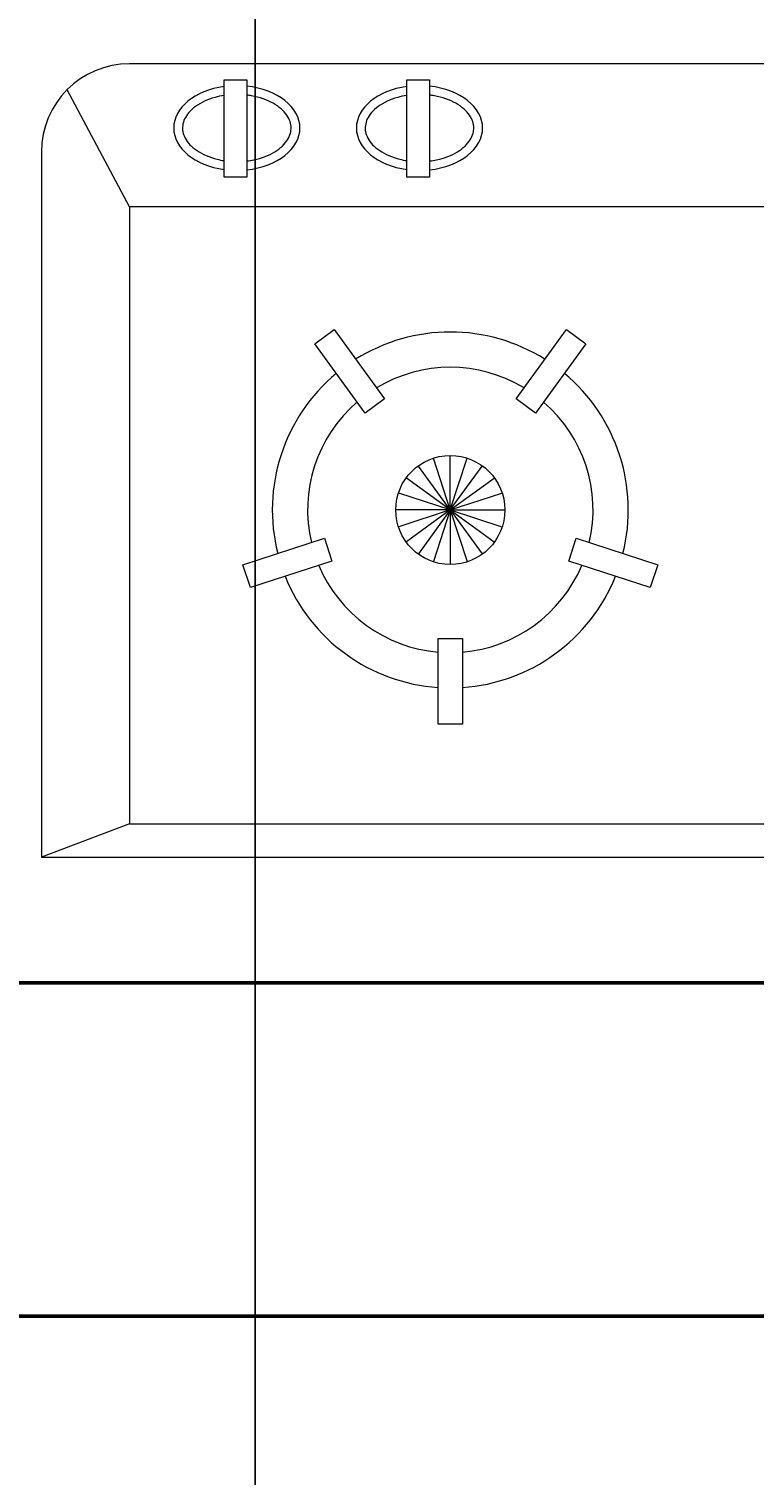
# Model space of a CAD drawing. Units: inches. Extents: x -173 to 545, y -746 to 104.
# Tile 10 of 32: x 300 to 320, y -702 to -663. Entities that reach past the tile are written whole.
import ezdxf

# ---------------------------------------------------------------- set-up
doc = ezdxf.new("R2010")
doc.units = ezdxf.units.IN
doc.header["$MEASUREMENT"] = 0
for name, color, linetype, lineweight in [('A-ANNO-DIMS', 2, 'Continuous', 18), ('A-EQPM', 8, 'Continuous', 18), ('A-WALL', 7, 'Continuous', 50)]:
    doc.layers.add(name, color=color, linetype=linetype, lineweight=lineweight)
doc.styles.get("Standard").update_dxf_attribs({"font": 'arial.ttf'})
doc.dimstyles.get("Standard").update_dxf_attribs({"dimtxt": 0.18, "dimasz": 0.18, "dimexe": 0.18, "dimexo": 0.0625, "dimgap": 0.09, "dimtad": 0, "dimtih": 1, "dimtoh": 1, "dimdec": 0, "dimzin": 0, "dimdsep": 46, "dimlunit": 3, "dimtxsty": 'Standard', "dimcen": 0.09, "dimadec": 0, "dimazin": 0, "dimtfac": 1, "dimtdec": 0, "dimtofl": 0, "dimtmove": 0, "dimatfit": 3, "dimfxl": 1, "dimtolj": 1, "dimtzin": 0, "dimarcsym": 0})

# ---------------------------------------------------------------- blocks, each defined once
blk = doc.blocks.new('HOB-38-BURNER')
for p, q in [((1.939, 10.273), (2.465, 10.656)), ((2.465, 10.656), (3.825, 8.784)), ((7.38, 8.784), (8.739, 10.656)), ((8.739, 10.656), (9.265, 10.273)), ((3.299, 8.402), (1.939, 10.273)), ((9.265, 10.273), (7.906, 8.402)), ((3.825, 8.784), (3.299, 8.402)), ((7.906, 8.402), (7.38, 8.784)), ((5.602, 5.784), (5.149, 7.18)), ((5.602, 5.784), (5.602, 7.251)), ((5.602, 5.784), (6.056, 7.18)), ((5.602, 5.784), (4.415, 6.647)), ((5.602, 5.784), (4.74, 6.971)), ((5.602, 5.784), (6.465, 6.971)), ((5.602, 5.784), (6.789, 6.647)), ((5.602, 5.784), (4.207, 6.238)), ((5.602, 5.784), (6.997, 6.238)), ((5.602, 5.784), (4.135, 5.784)), ((5.602, 5.784), (4.207, 5.331)), ((5.602, 5.784), (4.415, 4.922)), ((5.602, 5.784), (4.74, 4.598)), ((5.602, 5.784), (5.149, 4.389)), ((5.602, 5.784), (7.069, 5.784)), ((5.602, 5.784), (6.997, 5.331)), ((5.602, 5.784), (6.789, 4.922)), ((5.602, 5.784), (6.465, 4.598)), ((5.602, 5.784), (6.056, 4.389)), ((5.602, 5.784), (5.602, 4.317)), ((0, 4.306), (2.2, 5.021)), ((2.2, 5.021), (2.401, 4.402)), ((8.804, 4.402), (9.005, 5.021)), ((9.005, 5.021), (11.204, 4.306)), ((0.201, 3.688), (0, 4.306)), ((2.401, 4.402), (0.201, 3.688)), ((11.003, 3.688), (8.804, 4.402)), ((11.204, 4.306), (11.003, 3.688)), ((5.277, 2.313), (5.927, 2.313)), ((5.277, 0), (5.277, 2.313)), ((5.927, 2.313), (5.927, 0)), ((5.927, 0), (5.277, 0))]:
    blk.add_line(p, q)
blk.add_circle((5.602, 5.784), 1.474)
for radius, start, end in [(4.808, 57.8765, 122.1235), (4.808, 129.8765, 194.1235), (3.855, 58.8365, 121.1635), (4.808, 345.8765, 50.1235), (3.855, 130.8365, 193.1635), (3.855, 346.8365, 49.1635), (4.808, 201.8765, 266.1235), (3.855, 202.8365, 265.1635), (3.855, 274.8365, 337.1635), (4.808, 273.8765, 338.1235)]:
    blk.add_arc((5.602, 5.784), radius, start, end)
blk = doc.blocks.new('*D81')
at = {"layer": 'A-ANNO-DIMS', "color": 0, "lineweight": -2, "transparency": 16777216}
for p, q in [((219.801, -551.924), (219.801, -740.642)), ((306.301, -551.924), (306.301, -740.642)), ((219.981, -740.462), (262.513, -740.462)), ((306.121, -740.462), (263.59, -740.462))]:
    blk.add_line(p, q, dxfattribs=at)
at = {"layer": 'A-ANNO-DIMS', "color": 0, "transparency": 16777216}
for points in [[(219.981, -740.432), (219.981, -740.492), (219.801, -740.462)], [(306.121, -740.432), (306.121, -740.492), (306.301, -740.462)]]:
    blk.add_solid(points, dxfattribs=at)
at = {"layer": 'Defpoints', "color": 0, "transparency": 16777216}
for p in [(219.801, -551.862), (306.301, -551.862), (306.301, -740.462)]:
    blk.add_point(p, dxfattribs=at)
at = {"layer": 'A-ANNO-DIMS', "color": 0, "transparency": 16777216, "insert": (263.051, -740.462), "char_height": 0.18, "attachment_point": 5}
blk.add_mtext('\\A1;7\'-2 1/2"', dxfattribs=at)

msp = doc.modelspace()

# ---------------------------------------------------------------- linework, layer by layer
at = {"layer": 'A-EQPM'}
for p, q in [((336.255, -663.529), (302.912, -663.529)), ((302.912, -667.388), (301.227, -664.227)), ((305.464, -666.593), (305.464, -663.958)), ((305.464, -663.958), (306.08, -663.958)), ((306.08, -663.958), (306.08, -666.593)), ((310.398, -666.593), (310.398, -663.958)), ((310.398, -663.958), (311.015, -663.958)), ((311.015, -663.958), (311.015, -666.593)), ((300.53, -665.911), (300.53, -684.964)), ((306.08, -666.593), (305.464, -666.593)), ((311.015, -666.593), (310.398, -666.593)), ((302.912, -667.388), (302.912, -684.059)), ((336.255, -667.388), (302.912, -667.388)), ((302.912, -684.059), (300.53, -684.964)), ((302.912, -684.059), (336.255, -684.059)), ((300.53, -684.964), (338.637, -684.964))]:
    msp.add_line(p, q, dxfattribs=at)
msp.add_arc((302.912, -665.911), 2.382, 90, 180, dxfattribs=at)
for centre, major_axis, start_param, end_param in [((305.809, -665.263), (1.705, 0), 1.774361, 4.508825), ((305.809, -665.263), (-1.705, 0), 1.73081, 4.552375), ((310.743, -665.263), (1.705, 0), 1.774361, 4.508825), ((310.743, -665.263), (-1.705, 0), 1.73081, 4.552375)]:
    msp.add_ellipse(centre, major_axis=major_axis, ratio=0.671641, start_param=start_param, end_param=end_param, dxfattribs=at)
for points, knots in [([(305.464, -664.383), (305.381, -664.395), (305.3, -664.413), (305.119, -664.463), (305.022, -664.499), (304.845, -664.582), (304.764, -664.629), (304.623, -664.732), (304.563, -664.788), (304.465, -664.902), (304.427, -664.961), (304.371, -665.077), (304.354, -665.135), (304.339, -665.251), (304.341, -665.308), (304.363, -665.423), (304.384, -665.482), (304.447, -665.598), (304.489, -665.657), (304.596, -665.769), (304.66, -665.824), (304.808, -665.924), (304.892, -665.969), (305.075, -666.048), (305.175, -666.081), (305.339, -666.122), (305.401, -666.134), (305.464, -666.144)], [8.079302, 8.079302, 8.079302, 8.079302, 8.245651, 8.245651, 8.463703, 8.463703, 8.681755, 8.681755, 8.899807, 8.899807, 9.117859, 9.117859, 9.33591, 9.33591, 9.553962, 9.553962, 9.772014, 9.772014, 9.990066, 9.990066, 10.208118, 10.208118, 10.426169, 10.426169, 10.644221, 10.644221, 10.770253, 10.770253, 10.770253, 10.770253]), ([(306.08, -666.154), (306.144, -666.146), (306.207, -666.136), (306.375, -666.101), (306.477, -666.071), (306.666, -665.998), (306.754, -665.954), (306.911, -665.859), (306.98, -665.806), (307.096, -665.695), (307.143, -665.637), (307.216, -665.521), (307.241, -665.462), (307.269, -665.357), (307.275, -665.31), (307.275, -665.263), (307.275, -665.206), (307.266, -665.148), (307.228, -665.032), (307.199, -664.973), (307.118, -664.857), (307.067, -664.8), (306.943, -664.691), (306.87, -664.64), (306.706, -664.548), (306.616, -664.507), (306.421, -664.439), (306.317, -664.411), (306.167, -664.384), (306.124, -664.378), (306.08, -664.373)], [4.889299, 4.889299, 4.889299, 4.889299, 5.015191, 5.015191, 5.233243, 5.233243, 5.451295, 5.451295, 5.669347, 5.669347, 5.887399, 5.887399, 6.10545, 6.10545, 6.283185, 6.283185, 6.283185, 6.501237, 6.501237, 6.719289, 6.719289, 6.937341, 6.937341, 7.155392, 7.155392, 7.373444, 7.373444, 7.591496, 7.591496, 7.677072, 7.677072, 7.677072, 7.677072]), ([(310.398, -664.383), (310.315, -664.395), (310.234, -664.413), (310.053, -664.463), (309.957, -664.499), (309.779, -664.582), (309.698, -664.629), (309.558, -664.732), (309.497, -664.788), (309.399, -664.902), (309.361, -664.961), (309.306, -665.077), (309.289, -665.135), (309.273, -665.251), (309.275, -665.308), (309.297, -665.423), (309.318, -665.482), (309.381, -665.598), (309.423, -665.657), (309.53, -665.769), (309.594, -665.824), (309.742, -665.924), (309.826, -665.969), (310.01, -666.048), (310.109, -666.081), (310.273, -666.122), (310.335, -666.134), (310.398, -666.144)], [8.079302, 8.079302, 8.079302, 8.079302, 8.245651, 8.245651, 8.463703, 8.463703, 8.681755, 8.681755, 8.899807, 8.899807, 9.117859, 9.117859, 9.33591, 9.33591, 9.553962, 9.553962, 9.772014, 9.772014, 9.990066, 9.990066, 10.208118, 10.208118, 10.426169, 10.426169, 10.644221, 10.644221, 10.770253, 10.770253, 10.770253, 10.770253]), ([(311.015, -666.154), (311.078, -666.146), (311.141, -666.136), (311.309, -666.101), (311.411, -666.071), (311.601, -665.998), (311.688, -665.954), (311.845, -665.859), (311.914, -665.806), (312.03, -665.695), (312.078, -665.637), (312.15, -665.521), (312.175, -665.462), (312.203, -665.357), (312.21, -665.31), (312.21, -665.263), (312.21, -665.206), (312.2, -665.148), (312.162, -665.032), (312.133, -664.973), (312.052, -664.857), (312.001, -664.8), (311.877, -664.691), (311.804, -664.64), (311.641, -664.548), (311.55, -664.507), (311.355, -664.439), (311.251, -664.411), (311.101, -664.384), (311.058, -664.378), (311.015, -664.373)], [4.889299, 4.889299, 4.889299, 4.889299, 5.015191, 5.015191, 5.233243, 5.233243, 5.451295, 5.451295, 5.669347, 5.669347, 5.887399, 5.887399, 6.10545, 6.10545, 6.283185, 6.283185, 6.283185, 6.501237, 6.501237, 6.719289, 6.719289, 6.937341, 6.937341, 7.155392, 7.155392, 7.373444, 7.373444, 7.591496, 7.591496, 7.677072, 7.677072, 7.677072, 7.677072])]:
    msp.add_open_spline(points, degree=3, knots=knots, dxfattribs=at)
at = {"layer": 'A-WALL'}
for p, q in [((265.301, -688.362), (356.301, -688.362)), ((24.301, -697.362), (501.801, -697.362))]:
    msp.add_line(p, q, dxfattribs=at)

# ---------------------------------------------------------------- block references
at = {"layer": 'A-EQPM'}
msp.add_blockref('HOB-38-BURNER', (305.973, -681.367), dxfattribs=at)

# ---------------------------------------------------------------- dimensions: what is measured, and where the dimension line sits
at = {"layer": 'A-ANNO-DIMS'}
dim = msp.add_linear_dim(base=(306.301, -740.462), p1=(219.801, -551.862), p2=(306.301, -551.862), dimstyle='Standard', override={"dimdec": 1, "dimlfac": 1, "dimrnd": 0, "dimzin": 1, "dimdsep": 46, "dimlunit": 4, "dimfrac": 2}, dxfattribs=at)
dim.commit()
dim.dimension.update_dxf_attribs({"geometry": '*D81', "text_midpoint": (263.051, -740.462)})

doc.saveas('drawing.dxf')
